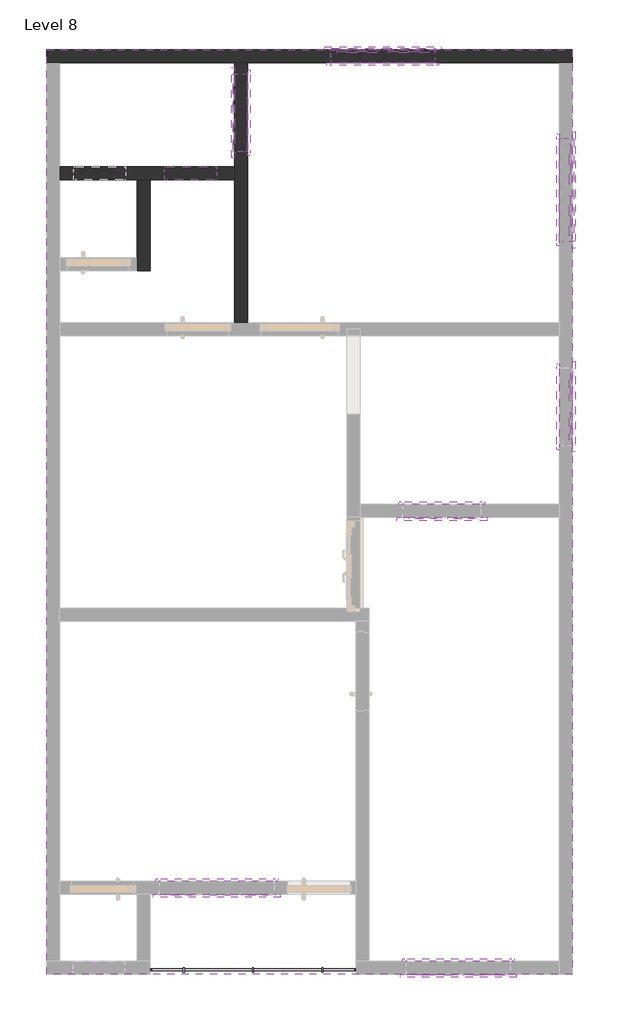
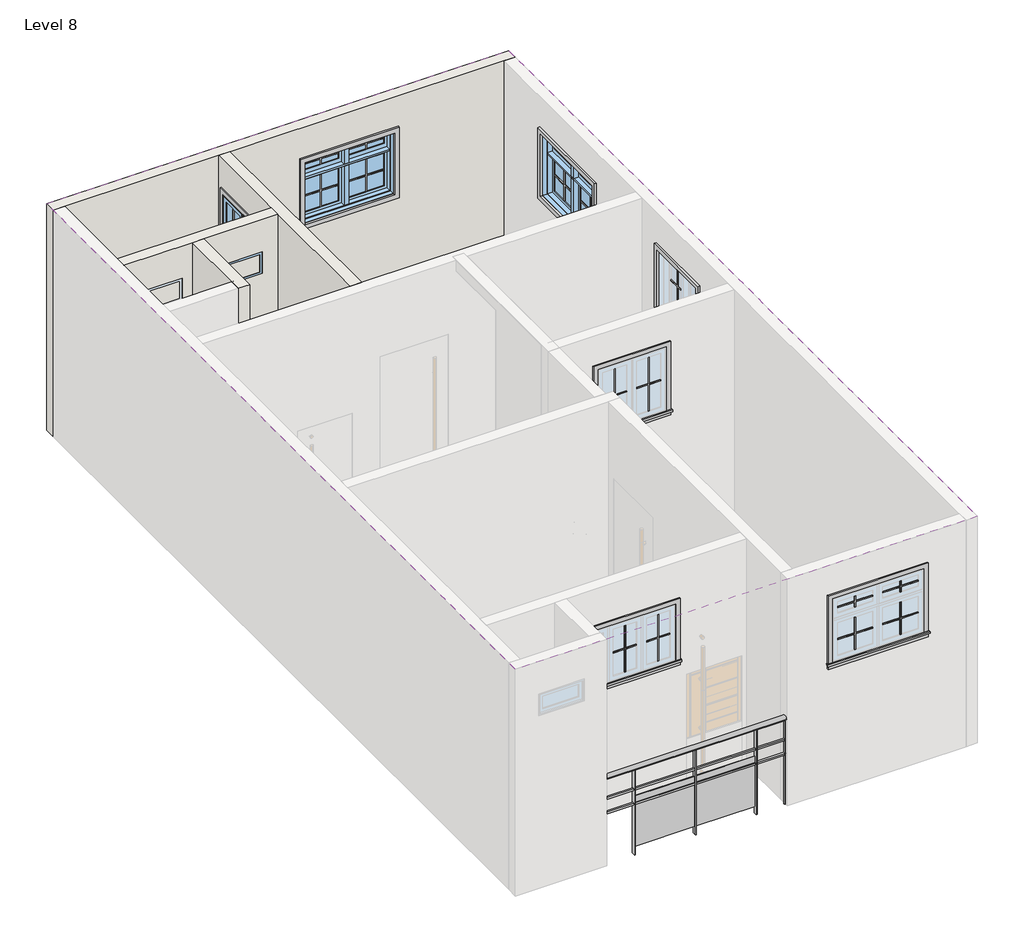
# One storey, part 2 of 2: 48 proxies, 7 walls, 5 windows, 1 covering, 1 railing.
"""IFC4 building model written with IfcOpenShell, lengths in millimetres."""

from ifc_helpers import new_model, si_unit, point, frame, origin, place, context, project, spatial, polyline, ellipse_curve, trimmed, outline, extrude, faceted_brep, transform, mapped, element, save
from ifc_brep_helpers import plane_surface, extruded_surface, advanced_brep
from components import m_muntin_pattern_2x2_m_muntin_pattern_2x2_ec2ff75e, m_muntin_pattern_2x2_m_muntin_pattern_2x2_6a19bea2, m_muntin_pattern_2x2_m_muntin_pattern_2x2_383df7b3, m_muntin_pattern_2x2_m_muntin_pattern_2x2_55460d9e, m_muntin_pattern_2x2_m_muntin_pattern_2x2_a9b7b7a9, m_muntin_pattern_2x2_m_muntin_pattern_2x2_c959817e, m_muntin_pattern_2x2_m_muntin_pattern_2x2_9259c5e2, m_trim_window_exterior_flat_with_sill_b1b88069, m_trim_window_exterior_flat_with_sill_8fa486dc, m_trim_window_exterior_flat_with_sill_2a9c44ae, m_trim_window_interior_flat_picture_frame_7d12f20c, m_trim_window_interior_flat_picture_frame_b6dd03a6, m_trim_window_interior_flat_picture_frame_c139440e, fixed_2_65c13adb, m_window_casement_double_3_e0bd8fa3, m_window_casement_double_awning_double_4_7efa9bbd

model = new_model("IFC4")

# Units and contexts
model_context = context("Model", 3, world=origin())
ifc_project = project(units=[si_unit("LENGTHUNIT", "METRE", prefix="MILLI")], contexts=[model_context])

# Site, building, storey
site = spatial("IfcSite", under=ifc_project)
building = spatial("IfcBuilding", under=site)
storey = spatial("IfcBuildingStorey", under=building, Name="Level 8", Elevation=13411.2)

# Proxies
placement = place(None, origin())
m_muntin_pattern_2x2_m_muntin_pattern_2x2_shape = m_muntin_pattern_2x2_m_muntin_pattern_2x2_ec2ff75e(model_context)
element("IfcBuildingElementProxy", 1, Name="M_Muntin Pattern_2x2 : M_Muntin Pattern_2x2", ObjectType="M_Muntin Pattern_2x2 : M_Muntin Pattern_2x2", at=placement, inside=storey, context=model_context, shape_type="MappedRepresentation", body=[
    mapped(m_muntin_pattern_2x2_m_muntin_pattern_2x2_shape, transform((-20164.8088079, 6316.5492053, 15309.85), x_axis=(1.0, 0.0, 0.0), y_axis=(0.0, 1.0, 0.0), z_axis=(0.0, 0.0, 1.0))),
])
element("IfcBuildingElementProxy", 2, Name="M_Muntin Pattern_2x2 : M_Muntin Pattern_2x2", ObjectType="M_Muntin Pattern_2x2 : M_Muntin Pattern_2x2", at=placement, inside=storey, context=model_context, shape_type="MappedRepresentation", body=[
    mapped(m_muntin_pattern_2x2_m_muntin_pattern_2x2_shape, transform((-17648.6213079, 4984.6367053, 15309.85), x_axis=(0.0, -1.0, 0.0), y_axis=(1.0, 0.0, 0.0), z_axis=(0.0, 0.0, 1.0))),
])
element("IfcBuildingElementProxy", 3, Name="M_Muntin Pattern_2x2 : M_Muntin Pattern_2x2", ObjectType="M_Muntin Pattern_2x2 : M_Muntin Pattern_2x2", at=placement, inside=storey, context=model_context, shape_type="MappedRepresentation", body=[
    mapped(m_muntin_pattern_2x2_m_muntin_pattern_2x2_shape, transform((-18672.7572454, -4510.2007947, 15309.85), x_axis=(-1.0, 0.0, 0.0), y_axis=(0.0, -1.0, 0.0), z_axis=(0.0, 0.0, 1.0))),
])
m_muntin_pattern_2x2_m_muntin_pattern_2x2_2_shape = m_muntin_pattern_2x2_m_muntin_pattern_2x2_6a19bea2(model_context)
element("IfcBuildingElementProxy", 4, Name="M_Muntin Pattern_2x2 : M_Muntin Pattern_2x2", ObjectType="M_Muntin Pattern_2x2 : M_Muntin Pattern_2x2", at=placement, inside=storey, context=model_context, shape_type="MappedRepresentation", body=[
    mapped(m_muntin_pattern_2x2_m_muntin_pattern_2x2_2_shape, transform((-19558.3838079, 6316.5492053, 15309.85), x_axis=(-1.0, 0.0, 0.0), y_axis=(0.0, -1.0, 0.0), z_axis=(0.0, 0.0, 1.0))),
])
element("IfcBuildingElementProxy", 5, Name="M_Muntin Pattern_2x2 : M_Muntin Pattern_2x2", ObjectType="M_Muntin Pattern_2x2 : M_Muntin Pattern_2x2", at=placement, inside=storey, context=model_context, shape_type="MappedRepresentation", body=[
    mapped(m_muntin_pattern_2x2_m_muntin_pattern_2x2_2_shape, transform((-17648.6213079, 4378.2117053, 15309.85), x_axis=(0.0, 1.0, 0.0), y_axis=(-1.0, 0.0, 0.0), z_axis=(0.0, 0.0, 1.0))),
])
element("IfcBuildingElementProxy", 6, Name="M_Muntin Pattern_2x2 : M_Muntin Pattern_2x2", ObjectType="M_Muntin Pattern_2x2 : M_Muntin Pattern_2x2", at=placement, inside=storey, context=model_context, shape_type="MappedRepresentation", body=[
    mapped(m_muntin_pattern_2x2_m_muntin_pattern_2x2_2_shape, transform((-19279.1822454, -4510.2007947, 15309.85), x_axis=(1.0, 0.0, 0.0), y_axis=(0.0, 1.0, 0.0), z_axis=(0.0, 0.0, 1.0))),
])
m_muntin_pattern_2x2_m_muntin_pattern_2x2_3_shape = m_muntin_pattern_2x2_m_muntin_pattern_2x2_383df7b3(model_context)
element("IfcBuildingElementProxy", 7, Name="M_Muntin Pattern_2x2 : M_Muntin Pattern_2x2", ObjectType="M_Muntin Pattern_2x2 : M_Muntin Pattern_2x2", at=placement, inside=storey, context=model_context, shape_type="MappedRepresentation", body=[
    mapped(m_muntin_pattern_2x2_m_muntin_pattern_2x2_3_shape, transform((-19558.3838079, 6316.5492053, 15909.85), x_axis=(-1.0, 0.0, 0.0), y_axis=(0.0, -1.0, 0.0), z_axis=(0.0, 0.0, 1.0))),
])
element("IfcBuildingElementProxy", 8, Name="M_Muntin Pattern_2x2 : M_Muntin Pattern_2x2", ObjectType="M_Muntin Pattern_2x2 : M_Muntin Pattern_2x2", at=placement, inside=storey, context=model_context, shape_type="MappedRepresentation", body=[
    mapped(m_muntin_pattern_2x2_m_muntin_pattern_2x2_3_shape, transform((-20164.8088079, 6316.5492053, 15909.85), x_axis=(-1.0, 0.0, 0.0), y_axis=(0.0, -1.0, 0.0), z_axis=(0.0, 0.0, 1.0))),
])
element("IfcBuildingElementProxy", 9, Name="M_Muntin Pattern_2x2 : M_Muntin Pattern_2x2", ObjectType="M_Muntin Pattern_2x2 : M_Muntin Pattern_2x2", at=placement, inside=storey, context=model_context, shape_type="MappedRepresentation", body=[
    mapped(m_muntin_pattern_2x2_m_muntin_pattern_2x2_3_shape, transform((-17648.6213079, 4378.2117053, 15909.85), x_axis=(0.0, 1.0, 0.0), y_axis=(-1.0, 0.0, 0.0), z_axis=(0.0, 0.0, 1.0))),
])
element("IfcBuildingElementProxy", 10, Name="M_Muntin Pattern_2x2 : M_Muntin Pattern_2x2", ObjectType="M_Muntin Pattern_2x2 : M_Muntin Pattern_2x2", at=placement, inside=storey, context=model_context, shape_type="MappedRepresentation", body=[
    mapped(m_muntin_pattern_2x2_m_muntin_pattern_2x2_3_shape, transform((-17648.6213079, 4984.6367053, 15909.85), x_axis=(0.0, 1.0, 0.0), y_axis=(-1.0, 0.0, 0.0), z_axis=(0.0, 0.0, 1.0))),
])
element("IfcBuildingElementProxy", 11, Name="M_Muntin Pattern_2x2 : M_Muntin Pattern_2x2", ObjectType="M_Muntin Pattern_2x2 : M_Muntin Pattern_2x2", at=placement, inside=storey, context=model_context, shape_type="MappedRepresentation", body=[
    mapped(m_muntin_pattern_2x2_m_muntin_pattern_2x2_3_shape, transform((-19279.1822454, -4510.2007947, 15909.85), x_axis=(1.0, 0.0, 0.0), y_axis=(0.0, 1.0, 0.0), z_axis=(0.0, 0.0, 1.0))),
])
element("IfcBuildingElementProxy", 12, Name="M_Muntin Pattern_2x2 : M_Muntin Pattern_2x2", ObjectType="M_Muntin Pattern_2x2 : M_Muntin Pattern_2x2", at=placement, inside=storey, context=model_context, shape_type="MappedRepresentation", body=[
    mapped(m_muntin_pattern_2x2_m_muntin_pattern_2x2_3_shape, transform((-18672.7572454, -4510.2007947, 15909.85), x_axis=(1.0, 0.0, 0.0), y_axis=(0.0, 1.0, 0.0), z_axis=(0.0, 0.0, 1.0))),
])
m_muntin_pattern_2x2_m_muntin_pattern_2x2_4_shape = m_muntin_pattern_2x2_m_muntin_pattern_2x2_55460d9e(model_context)
element("IfcBuildingElementProxy", 13, Name="M_Muntin Pattern_2x2 : M_Muntin Pattern_2x2", ObjectType="M_Muntin Pattern_2x2 : M_Muntin Pattern_2x2", at=placement, inside=storey, context=model_context, shape_type="MappedRepresentation", body=[
    mapped(m_muntin_pattern_2x2_m_muntin_pattern_2x2_4_shape, transform((-18939.9533391, 849.1992053, 15309.85), x_axis=(-1.0, 0.0, 0.0), y_axis=(0.0, -1.0, 0.0), z_axis=(0.0, 0.0, 1.0))),
])
element("IfcBuildingElementProxy", 14, Name="M_Muntin Pattern_2x2 : M_Muntin Pattern_2x2", ObjectType="M_Muntin Pattern_2x2 : M_Muntin Pattern_2x2", at=placement, inside=storey, context=model_context, shape_type="MappedRepresentation", body=[
    mapped(m_muntin_pattern_2x2_m_muntin_pattern_2x2_4_shape, transform((-17648.6213079, 2366.8492053, 15309.85), x_axis=(0.0, -1.0, 0.0), y_axis=(1.0, 0.0, 0.0), z_axis=(0.0, 0.0, 1.0))),
])
element("IfcBuildingElementProxy", 15, Name="M_Muntin Pattern_2x2 : M_Muntin Pattern_2x2", ObjectType="M_Muntin Pattern_2x2 : M_Muntin Pattern_2x2", at=placement, inside=storey, context=model_context, shape_type="MappedRepresentation", body=[
    mapped(m_muntin_pattern_2x2_m_muntin_pattern_2x2_4_shape, transform((-21591.9713079, 5362.4617053, 15309.85), x_axis=(0.0, 1.0, 0.0), y_axis=(-1.0, 0.0, 0.0), z_axis=(0.0, 0.0, 1.0))),
])
element("IfcBuildingElementProxy", 16, Name="M_Muntin Pattern_2x2 : M_Muntin Pattern_2x2", ObjectType="M_Muntin Pattern_2x2 : M_Muntin Pattern_2x2", at=placement, inside=storey, context=model_context, shape_type="MappedRepresentation", body=[
    mapped(m_muntin_pattern_2x2_m_muntin_pattern_2x2_4_shape, transform((-18939.9533391, 849.1992053, 15309.85), x_axis=(-1.0, 0.0, 0.0), y_axis=(0.0, -1.0, 0.0), z_axis=(0.0, 0.0, 1.0))),
])
element("IfcBuildingElementProxy", 17, Name="M_Muntin Pattern_2x2 : M_Muntin Pattern_2x2", ObjectType="M_Muntin Pattern_2x2 : M_Muntin Pattern_2x2", at=placement, inside=storey, context=model_context, shape_type="MappedRepresentation", body=[
    mapped(m_muntin_pattern_2x2_m_muntin_pattern_2x2_4_shape, transform((-21591.9713079, 5362.4617053, 15309.85), x_axis=(0.0, 1.0, 0.0), y_axis=(-1.0, 0.0, 0.0), z_axis=(0.0, 0.0, 1.0))),
])
m_muntin_pattern_2x2_m_muntin_pattern_2x2_5_shape = m_muntin_pattern_2x2_m_muntin_pattern_2x2_a9b7b7a9(model_context)
element("IfcBuildingElementProxy", 18, Name="M_Muntin Pattern_2x2 : M_Muntin Pattern_2x2", ObjectType="M_Muntin Pattern_2x2 : M_Muntin Pattern_2x2", at=placement, inside=storey, context=model_context, shape_type="MappedRepresentation", body=[
    mapped(m_muntin_pattern_2x2_m_muntin_pattern_2x2_5_shape, transform((-19393.9783391, 849.1992053, 15309.85), x_axis=(1.0, 0.0, 0.0), y_axis=(0.0, 1.0, 0.0), z_axis=(0.0, 0.0, 1.0))),
])
element("IfcBuildingElementProxy", 19, Name="M_Muntin Pattern_2x2 : M_Muntin Pattern_2x2", ObjectType="M_Muntin Pattern_2x2 : M_Muntin Pattern_2x2", at=placement, inside=storey, context=model_context, shape_type="MappedRepresentation", body=[
    mapped(m_muntin_pattern_2x2_m_muntin_pattern_2x2_5_shape, transform((-17648.6213079, 1912.8242053, 15309.85), x_axis=(0.0, 1.0, 0.0), y_axis=(-1.0, 0.0, 0.0), z_axis=(0.0, 0.0, 1.0))),
])
element("IfcBuildingElementProxy", 20, Name="M_Muntin Pattern_2x2 : M_Muntin Pattern_2x2", ObjectType="M_Muntin Pattern_2x2 : M_Muntin Pattern_2x2", at=placement, inside=storey, context=model_context, shape_type="MappedRepresentation", body=[
    mapped(m_muntin_pattern_2x2_m_muntin_pattern_2x2_5_shape, transform((-21591.9713079, 5816.4867053, 15309.85), x_axis=(0.0, -1.0, 0.0), y_axis=(1.0, 0.0, 0.0), z_axis=(0.0, 0.0, 1.0))),
])
element("IfcBuildingElementProxy", 21, Name="M_Muntin Pattern_2x2 : M_Muntin Pattern_2x2", ObjectType="M_Muntin Pattern_2x2 : M_Muntin Pattern_2x2", at=placement, inside=storey, context=model_context, shape_type="MappedRepresentation", body=[
    mapped(m_muntin_pattern_2x2_m_muntin_pattern_2x2_5_shape, transform((-19393.9783391, 849.1992053, 15309.85), x_axis=(1.0, 0.0, 0.0), y_axis=(0.0, 1.0, 0.0), z_axis=(0.0, 0.0, 1.0))),
])
element("IfcBuildingElementProxy", 22, Name="M_Muntin Pattern_2x2 : M_Muntin Pattern_2x2", ObjectType="M_Muntin Pattern_2x2 : M_Muntin Pattern_2x2", at=placement, inside=storey, context=model_context, shape_type="MappedRepresentation", body=[
    mapped(m_muntin_pattern_2x2_m_muntin_pattern_2x2_5_shape, transform((-21591.9713079, 5816.4867053, 15309.85), x_axis=(0.0, -1.0, 0.0), y_axis=(1.0, 0.0, 0.0), z_axis=(0.0, 0.0, 1.0))),
])
m_muntin_pattern_2x2_m_muntin_pattern_2x2_6_shape = m_muntin_pattern_2x2_m_muntin_pattern_2x2_c959817e(model_context)
element("IfcBuildingElementProxy", 23, Name="M_Muntin Pattern_2x2 : M_Muntin Pattern_2x2", ObjectType="M_Muntin Pattern_2x2 : M_Muntin Pattern_2x2", at=placement, inside=storey, context=model_context, shape_type="MappedRepresentation", body=[
    mapped(m_muntin_pattern_2x2_m_muntin_pattern_2x2_6_shape, transform((-21364.4296412, -3570.4007947, 15309.85), x_axis=(-1.0, 0.0, 0.0), y_axis=(0.0, -1.0, 0.0), z_axis=(0.0, 0.0, 1.0))),
])
element("IfcBuildingElementProxy", 24, Name="M_Muntin Pattern_2x2 : M_Muntin Pattern_2x2", ObjectType="M_Muntin Pattern_2x2 : M_Muntin Pattern_2x2", at=placement, inside=storey, context=model_context, shape_type="MappedRepresentation", body=[
    mapped(m_muntin_pattern_2x2_m_muntin_pattern_2x2_6_shape, transform((-21364.4296412, -3570.4007947, 15309.85), x_axis=(-1.0, 0.0, 0.0), y_axis=(0.0, -1.0, 0.0), z_axis=(0.0, 0.0, 1.0))),
])
m_muntin_pattern_2x2_m_muntin_pattern_2x2_7_shape = m_muntin_pattern_2x2_m_muntin_pattern_2x2_9259c5e2(model_context)
element("IfcBuildingElementProxy", 25, Name="M_Muntin Pattern_2x2 : M_Muntin Pattern_2x2", ObjectType="M_Muntin Pattern_2x2 : M_Muntin Pattern_2x2", at=placement, inside=storey, context=model_context, shape_type="MappedRepresentation", body=[
    mapped(m_muntin_pattern_2x2_m_muntin_pattern_2x2_7_shape, transform((-22257.6629746, -3570.4007947, 15309.85), x_axis=(1.0, 0.0, 0.0), y_axis=(0.0, 1.0, 0.0), z_axis=(0.0, 0.0, 1.0))),
])
element("IfcBuildingElementProxy", 26, Name="M_Muntin Pattern_2x2 : M_Muntin Pattern_2x2", ObjectType="M_Muntin Pattern_2x2 : M_Muntin Pattern_2x2", at=placement, inside=storey, context=model_context, shape_type="MappedRepresentation", body=[
    mapped(m_muntin_pattern_2x2_m_muntin_pattern_2x2_7_shape, transform((-21811.0463079, -3570.4007947, 15309.85), x_axis=(1.0, 0.0, 0.0), y_axis=(0.0, 1.0, 0.0), z_axis=(0.0, 0.0, 1.0))),
])
element("IfcBuildingElementProxy", 27, Name="M_Muntin Pattern_2x2 : M_Muntin Pattern_2x2", ObjectType="M_Muntin Pattern_2x2 : M_Muntin Pattern_2x2", at=placement, inside=storey, context=model_context, shape_type="MappedRepresentation", body=[
    mapped(m_muntin_pattern_2x2_m_muntin_pattern_2x2_7_shape, transform((-22257.6629746, -3570.4007947, 15309.85), x_axis=(1.0, 0.0, 0.0), y_axis=(0.0, 1.0, 0.0), z_axis=(0.0, 0.0, 1.0))),
])
element("IfcBuildingElementProxy", 28, Name="M_Muntin Pattern_2x2 : M_Muntin Pattern_2x2", ObjectType="M_Muntin Pattern_2x2 : M_Muntin Pattern_2x2", at=placement, inside=storey, context=model_context, shape_type="MappedRepresentation", body=[
    mapped(m_muntin_pattern_2x2_m_muntin_pattern_2x2_7_shape, transform((-21811.0463079, -3570.4007947, 15309.85), x_axis=(1.0, 0.0, 0.0), y_axis=(0.0, 1.0, 0.0), z_axis=(0.0, 0.0, 1.0))),
])
m_trim_window_exterior_flat_with_sill_shape = m_trim_window_exterior_flat_with_sill_b1b88069(model_context)
element("IfcBuildingElementProxy", 29, Name="M_Trim-Window-Exterior-Flat : with Sill", ObjectType="M_Trim-Window-Exterior-Flat : with Sill", at=placement, inside=storey, context=model_context, shape_type="MappedRepresentation", body=[
    mapped(m_trim_window_exterior_flat_with_sill_shape, transform((-19861.5963079, 6326.0742053, 16140.0), x_axis=(-1.0, 0.0, 0.0), y_axis=(0.0, 0.0, 1.0), z_axis=(0.0, 1.0, 0.0))),
])
element("IfcBuildingElementProxy", 30, Name="M_Trim-Window-Exterior-Flat : with Sill", ObjectType="M_Trim-Window-Exterior-Flat : with Sill", at=placement, inside=storey, context=model_context, shape_type="MappedRepresentation", body=[
    mapped(m_trim_window_exterior_flat_with_sill_shape, transform((-17639.0963079, 4681.4242053, 16140.0), x_axis=(0.0, 1.0, 0.0), y_axis=(0.0, 0.0, 1.0), z_axis=(1.0, 0.0, 0.0))),
])
element("IfcBuildingElementProxy", 31, Name="M_Trim-Window-Exterior-Flat : with Sill", ObjectType="M_Trim-Window-Exterior-Flat : with Sill", at=placement, inside=storey, context=model_context, shape_type="MappedRepresentation", body=[
    mapped(m_trim_window_exterior_flat_with_sill_shape, transform((-18975.9697454, -4519.7257947, 16140.0), x_axis=(1.0, 0.0, 0.0), y_axis=(0.0, 0.0, 1.0), z_axis=(0.0, -1.0, 0.0))),
])
m_trim_window_exterior_flat_with_sill_2_shape = m_trim_window_exterior_flat_with_sill_8fa486dc(model_context)
element("IfcBuildingElementProxy", 32, Name="M_Trim-Window-Exterior-Flat : with Sill", ObjectType="M_Trim-Window-Exterior-Flat : with Sill", at=placement, inside=storey, context=model_context, shape_type="MappedRepresentation", body=[
    mapped(m_trim_window_exterior_flat_with_sill_2_shape, transform((-19166.9658391, 839.6742053, 16140.0), x_axis=(1.0, 0.0, 0.0), y_axis=(0.0, 0.0, 1.0), z_axis=(0.0, -1.0, 0.0))),
])
element("IfcBuildingElementProxy", 33, Name="M_Trim-Window-Exterior-Flat : with Sill", ObjectType="M_Trim-Window-Exterior-Flat : with Sill", at=placement, inside=storey, context=model_context, shape_type="MappedRepresentation", body=[
    mapped(m_trim_window_exterior_flat_with_sill_2_shape, transform((-17639.0963079, 2139.8367053, 16140.0), x_axis=(0.0, 1.0, 0.0), y_axis=(0.0, 0.0, 1.0), z_axis=(1.0, 0.0, 0.0))),
])
element("IfcBuildingElementProxy", 34, Name="M_Trim-Window-Exterior-Flat : with Sill", ObjectType="M_Trim-Window-Exterior-Flat : with Sill", at=placement, inside=storey, context=model_context, shape_type="MappedRepresentation", body=[
    mapped(m_trim_window_exterior_flat_with_sill_2_shape, transform((-21601.4963079, 5589.4742053, 16140.0), x_axis=(0.0, -1.0, 0.0), y_axis=(0.0, 0.0, 1.0), z_axis=(-1.0, 0.0, 0.0))),
])
element("IfcBuildingElementProxy", 35, Name="M_Trim-Window-Exterior-Flat : with Sill", ObjectType="M_Trim-Window-Exterior-Flat : with Sill", at=placement, inside=storey, context=model_context, shape_type="MappedRepresentation", body=[
    mapped(m_trim_window_exterior_flat_with_sill_2_shape, transform((-19166.9658391, 839.6742053, 16140.0), x_axis=(1.0, 0.0, 0.0), y_axis=(0.0, 0.0, 1.0), z_axis=(0.0, -1.0, 0.0))),
])
element("IfcBuildingElementProxy", 36, Name="M_Trim-Window-Exterior-Flat : with Sill", ObjectType="M_Trim-Window-Exterior-Flat : with Sill", at=placement, inside=storey, context=model_context, shape_type="MappedRepresentation", body=[
    mapped(m_trim_window_exterior_flat_with_sill_2_shape, transform((-21601.4963079, 5589.4742053, 16140.0), x_axis=(0.0, -1.0, 0.0), y_axis=(0.0, 0.0, 1.0), z_axis=(-1.0, 0.0, 0.0))),
])
m_trim_window_exterior_flat_with_sill_3_shape = m_trim_window_exterior_flat_with_sill_2a9c44ae(model_context)
element("IfcBuildingElementProxy", 37, Name="M_Trim-Window-Exterior-Flat : with Sill", ObjectType="M_Trim-Window-Exterior-Flat : with Sill", at=placement, inside=storey, context=model_context, shape_type="MappedRepresentation", body=[
    mapped(m_trim_window_exterior_flat_with_sill_3_shape, transform((-21811.0463079, -3579.9257947, 16040.0), x_axis=(1.0, 0.0, 0.0), y_axis=(0.0, 0.0, 1.0), z_axis=(0.0, -1.0, 0.0))),
])
element("IfcBuildingElementProxy", 38, Name="M_Trim-Window-Exterior-Flat : with Sill", ObjectType="M_Trim-Window-Exterior-Flat : with Sill", at=placement, inside=storey, context=model_context, shape_type="MappedRepresentation", body=[
    mapped(m_trim_window_exterior_flat_with_sill_3_shape, transform((-21811.0463079, -3579.9257947, 16040.0), x_axis=(1.0, 0.0, 0.0), y_axis=(0.0, 0.0, 1.0), z_axis=(0.0, -1.0, 0.0))),
])
m_trim_window_interior_flat_picture_frame_shape = m_trim_window_interior_flat_picture_frame_7d12f20c(model_context)
element("IfcBuildingElementProxy", 39, Name="M_Trim-Window-Interior-Flat : Picture Frame", ObjectType="M_Trim-Window-Interior-Flat : Picture Frame", at=placement, inside=storey, context=model_context, shape_type="MappedRepresentation", body=[
    mapped(m_trim_window_interior_flat_picture_frame_shape, transform((-19861.5963079, 6173.6742053, 16140.0), x_axis=(1.0, 0.0, 0.0), y_axis=(0.0, 0.0, 1.0), z_axis=(0.0, -1.0, 0.0))),
])
element("IfcBuildingElementProxy", 40, Name="M_Trim-Window-Interior-Flat : Picture Frame", ObjectType="M_Trim-Window-Interior-Flat : Picture Frame", at=placement, inside=storey, context=model_context, shape_type="MappedRepresentation", body=[
    mapped(m_trim_window_interior_flat_picture_frame_shape, transform((-17791.4963079, 4681.4242053, 16140.0), x_axis=(0.0, -1.0, 0.0), y_axis=(0.0, 0.0, 1.0), z_axis=(-1.0, 0.0, 0.0))),
])
element("IfcBuildingElementProxy", 41, Name="M_Trim-Window-Interior-Flat : Picture Frame", ObjectType="M_Trim-Window-Interior-Flat : Picture Frame", at=placement, inside=storey, context=model_context, shape_type="MappedRepresentation", body=[
    mapped(m_trim_window_interior_flat_picture_frame_shape, transform((-18975.9697454, -4367.3257947, 16140.0), x_axis=(-1.0, 0.0, 0.0), y_axis=(0.0, 0.0, 1.0), z_axis=(0.0, 1.0, 0.0))),
])
m_trim_window_interior_flat_picture_frame_2_shape = m_trim_window_interior_flat_picture_frame_b6dd03a6(model_context)
element("IfcBuildingElementProxy", 42, Name="M_Trim-Window-Interior-Flat : Picture Frame", ObjectType="M_Trim-Window-Interior-Flat : Picture Frame", at=placement, inside=storey, context=model_context, shape_type="MappedRepresentation", body=[
    mapped(m_trim_window_interior_flat_picture_frame_2_shape, transform((-19166.9658391, 992.0742053, 16140.0), x_axis=(-1.0, 0.0, 0.0), y_axis=(0.0, 0.0, 1.0), z_axis=(0.0, 1.0, 0.0))),
])
element("IfcBuildingElementProxy", 43, Name="M_Trim-Window-Interior-Flat : Picture Frame", ObjectType="M_Trim-Window-Interior-Flat : Picture Frame", at=placement, inside=storey, context=model_context, shape_type="MappedRepresentation", body=[
    mapped(m_trim_window_interior_flat_picture_frame_2_shape, transform((-17791.4963079, 2139.8367053, 16140.0), x_axis=(0.0, -1.0, 0.0), y_axis=(0.0, 0.0, 1.0), z_axis=(-1.0, 0.0, 0.0))),
])
element("IfcBuildingElementProxy", 44, Name="M_Trim-Window-Interior-Flat : Picture Frame", ObjectType="M_Trim-Window-Interior-Flat : Picture Frame", at=placement, inside=storey, context=model_context, shape_type="MappedRepresentation", body=[
    mapped(m_trim_window_interior_flat_picture_frame_2_shape, transform((-21449.0963079, 5589.4742053, 16140.0), x_axis=(0.0, 1.0, 0.0), y_axis=(0.0, 0.0, 1.0), z_axis=(1.0, 0.0, 0.0))),
])
element("IfcBuildingElementProxy", 45, Name="M_Trim-Window-Interior-Flat : Picture Frame", ObjectType="M_Trim-Window-Interior-Flat : Picture Frame", at=placement, inside=storey, context=model_context, shape_type="MappedRepresentation", body=[
    mapped(m_trim_window_interior_flat_picture_frame_2_shape, transform((-19166.9658391, 992.0742053, 16140.0), x_axis=(-1.0, 0.0, 0.0), y_axis=(0.0, 0.0, 1.0), z_axis=(0.0, 1.0, 0.0))),
])
element("IfcBuildingElementProxy", 46, Name="M_Trim-Window-Interior-Flat : Picture Frame", ObjectType="M_Trim-Window-Interior-Flat : Picture Frame", at=placement, inside=storey, context=model_context, shape_type="MappedRepresentation", body=[
    mapped(m_trim_window_interior_flat_picture_frame_2_shape, transform((-21449.0963079, 5589.4742053, 16140.0), x_axis=(0.0, 1.0, 0.0), y_axis=(0.0, 0.0, 1.0), z_axis=(1.0, 0.0, 0.0))),
])
m_trim_window_interior_flat_picture_frame_3_shape = m_trim_window_interior_flat_picture_frame_c139440e(model_context)
element("IfcBuildingElementProxy", 47, Name="M_Trim-Window-Interior-Flat : Picture Frame", ObjectType="M_Trim-Window-Interior-Flat : Picture Frame", at=placement, inside=storey, context=model_context, shape_type="MappedRepresentation", body=[
    mapped(m_trim_window_interior_flat_picture_frame_3_shape, transform((-21811.0463079, -3427.5257947, 16040.0), x_axis=(-1.0, 0.0, 0.0), y_axis=(0.0, 0.0, 1.0), z_axis=(0.0, 1.0, 0.0))),
])
element("IfcBuildingElementProxy", 48, Name="M_Trim-Window-Interior-Flat : Picture Frame", ObjectType="M_Trim-Window-Interior-Flat : Picture Frame", at=placement, inside=storey, context=model_context, shape_type="MappedRepresentation", body=[
    mapped(m_trim_window_interior_flat_picture_frame_3_shape, transform((-21811.0463079, -3427.5257947, 16040.0), x_axis=(-1.0, 0.0, 0.0), y_axis=(0.0, 0.0, 1.0), z_axis=(0.0, 1.0, 0.0))),
])

# Covering
element("IfcCovering", 49, ObjectType="2' x 4' ACT System", at=placement, inside=storey, context=model_context, shape_type="SweptSolid", body=[
    extrude(outline(polyline([(-23811.2963079, -4519.7257947), (-23811.2963079, 6326.0742053), (-17639.0963079, 6326.0742053), (-17639.0963079, -4519.7257947), (-22309.2664727, -4519.7257947), (-23811.2963079, -4519.7257947)])), frame((0.0, 0.0, 16611.6), z_axis=(0.0, 0.0, 1.0), x_axis=(1.0, 0.0, 0.0)), (0.0, 0.0, 1.0), 57.15),
])

# Railing
element("IfcRailing", 50, ObjectType="Glass Panel - Bottom Fill", at=placement, inside=storey, context=model_context, shape_type="SolidModel", body=[
    advanced_brep(
    [(-22592.0963079, -4430.8257947, 14630.4), (-22592.0963079, -4507.0257947, 14630.4), (-20179.0963079, -4430.8257947, 14630.4), (-20179.0963079, -4507.0257947, 14630.4)],
    [
        (0, 1, ellipse_curve(frame((-22592.0963079, -4468.9257947, 14630.4), z_axis=(-1.0, 0.0, 0.0), x_axis=(0.0, -1.0, 0.0)), 38.1, 28.575)),
        (1, 0, ellipse_curve(frame((-22592.0963079, -4468.9257947, 14630.4), z_axis=(-1.0, 0.0, 0.0), x_axis=(0.0, -1.0, 0.0)), 38.1, 28.575)),
        (2, 3, ellipse_curve(frame((-20179.0963079, -4468.9257947, 14630.4), z_axis=(1.0, 0.0, 0.0), x_axis=(0.0, -1.0, 0.0)), 38.1, 28.575)),
        (3, 2, ellipse_curve(frame((-20179.0963079, -4468.9257947, 14630.4), z_axis=(1.0, 0.0, 0.0), x_axis=(0.0, -1.0, 0.0)), 38.1, 28.575)),
        (0, 2),
        (3, 1),
    ],
    [
        plane_surface(frame((-22592.0963079, -4468.9257947, 14630.4), z_axis=(-1.0, 0.0, 0.0), x_axis=(0.0, 1.0, 0.0))),
        plane_surface(frame((-20179.0963079, -4468.9257947, 14630.4), z_axis=(1.0, 0.0, 0.0), x_axis=(0.0, 1.0, 0.0))),
        extruded_surface(trimmed(ellipse_curve(frame((-20179.0963079, -4468.9257947, 14630.4), z_axis=(-1.0, 0.0, 0.0), x_axis=(0.0, -1.0, 0.0)), 38.1, 28.575), [point((-20179.0963079, -4430.8257947, 14630.4))], [point((-20179.0963079, -4507.0257947, 14630.4))], True, "CARTESIAN"), (-2413.0, 0.0, 0.0), 2413.0),
        extruded_surface(trimmed(ellipse_curve(frame((-20179.0963079, -4468.9257947, 14630.4), z_axis=(-1.0, 0.0, 0.0), x_axis=(0.0, -1.0, 0.0)), 38.1, 28.575), [point((-20179.0963079, -4507.0257947, 14630.4))], [point((-20179.0963079, -4430.8257947, 14630.4))], True, "CARTESIAN"), (-2413.0, 0.0, 0.0), 2413.0),
    ],
    [
        (0, [[1, 2]]),
        (1, [[3, 4]]),
        (2, [[-1, 5, -4, 6]]),
        (3, [[-2, -6, -3, -5]]),
    ],
),
    extrude(outline(polyline([(-22592.0963079, -4481.6257947), (-22592.0963079, -4456.2257947), (-20179.0963079, -4456.2257947), (-20179.0963079, -4481.6257947), (-22592.0963079, -4481.6257947)])), frame((0.0, 0.0, 14312.9), z_axis=(0.0, 0.0, 1.0), x_axis=(1.0, 0.0, 0.0)), (0.0, 0.0, 1.0), 25.4),
    extrude(outline(polyline([(-22592.0963079, -4481.6257947), (-22592.0963079, -4456.2257947), (-20179.0963079, -4456.2257947), (-20179.0963079, -4481.6257947), (-22592.0963079, -4481.6257947)])), frame((0.0, 0.0, 14109.7), z_axis=(0.0, 0.0, 1.0), x_axis=(1.0, 0.0, 0.0)), (0.0, 0.0, 1.0), 25.4),
    extrude(outline(polyline([(-20579.1463079, -4494.3257947), (-20579.1463079, -4443.5257947), (-20566.4463079, -4443.5257947), (-20566.4463079, -4494.3257947), (-20579.1463079, -4494.3257947)])), frame((0.0, 0.0, 13411.2), z_axis=(0.0, 0.0, 1.0), x_axis=(1.0, 0.0, 0.0)), (0.0, 0.0, 1.0), 1190.625),
    extrude(outline(polyline([(-21385.5963079, -4462.3906377), (-20572.7963079, -4462.3906377), (-20572.7963079, -4468.7406377), (-21385.5963079, -4468.7406377), (-21385.5963079, -4462.3906377)])), frame((0.0, 0.0, 13512.8), z_axis=(0.0, 0.0, 1.0), x_axis=(1.0, 0.0, 0.0)), (0.0, 0.0, 1.0), 711.2),
    extrude(outline(polyline([(-21391.9463079, -4494.3257947), (-21391.9463079, -4443.5257947), (-21379.2463079, -4443.5257947), (-21379.2463079, -4494.3257947), (-21391.9463079, -4494.3257947)])), frame((0.0, 0.0, 13411.2), z_axis=(0.0, 0.0, 1.0), x_axis=(1.0, 0.0, 0.0)), (0.0, 0.0, 1.0), 1190.625),
    extrude(outline(polyline([(-22198.3963079, -4462.3906377), (-21385.5963079, -4462.3906377), (-21385.5963079, -4468.7406377), (-22198.3963079, -4468.7406377), (-22198.3963079, -4462.3906377)])), frame((0.0, 0.0, 13512.8), z_axis=(0.0, 0.0, 1.0), x_axis=(1.0, 0.0, 0.0)), (0.0, 0.0, 1.0), 711.2),
    extrude(outline(polyline([(-22204.7463079, -4494.3257947), (-22204.7463079, -4443.5257947), (-22192.0463079, -4443.5257947), (-22192.0463079, -4494.3257947), (-22204.7463079, -4494.3257947)])), frame((0.0, 0.0, 13411.2), z_axis=(0.0, 0.0, 1.0), x_axis=(1.0, 0.0, 0.0)), (0.0, 0.0, 1.0), 1190.625),
    extrude(outline(polyline([(-20191.7963079, -4478.4507947), (-20191.7963079, -4459.4007947), (-20172.7463079, -4459.4007947), (-20172.7463079, -4478.4507947), (-20191.7963079, -4478.4507947)])), frame((0.0, 0.0, 13411.2), z_axis=(0.0, 0.0, 1.0), x_axis=(1.0, 0.0, 0.0)), (0.0, 0.0, 1.0), 1190.625),
    extrude(outline(polyline([(-22598.4463079, -4478.4507947), (-22598.4463079, -4459.4007947), (-22579.3963079, -4459.4007947), (-22579.3963079, -4478.4507947), (-22598.4463079, -4478.4507947)])), frame((0.0, 0.0, 13411.2), z_axis=(0.0, 0.0, 1.0), x_axis=(1.0, 0.0, 0.0)), (0.0, 0.0, 1.0), 1190.625),
])

# Walls
element("IfcWall", 51, ObjectType="Generic - 6\"", at=placement, inside=storey, context=model_context, shape_type="Brep", body=[
    faceted_brep([(-23811.2963079, 6173.6742053, 13411.2), (-23658.8963079, 6173.6742053, 13411.2), (-21601.4963079, 6173.6742053, 13411.2), (-21449.0963079, 6173.6742053, 13411.2), (-17791.4963079, 6173.6742053, 13411.2), (-17639.0963079, 6173.6742053, 13411.2), (-17639.0963079, 6173.6742053, 16611.6), (-17791.4963079, 6173.6742053, 16611.6), (-21449.0963079, 6173.6742053, 16611.6), (-21601.4963079, 6173.6742053, 16611.6), (-23658.8963079, 6173.6742053, 16611.6), (-23811.2963079, 6173.6742053, 16611.6), (-19251.9963079, 6173.6742053, 16140.0), (-19251.9963079, 6173.6742053, 15240.0), (-20471.1963079, 6173.6742053, 15240.0), (-20471.1963079, 6173.6742053, 16140.0), (-23811.2963079, 6326.0742053, 13411.2), (-23811.2963079, 6326.0742053, 16611.6), (-17639.0963079, 6326.0742053, 16611.6), (-17639.0963079, 6326.0742053, 13411.2), (-19251.9963079, 6326.0742053, 16140.0), (-20471.1963079, 6326.0742053, 16140.0), (-20471.1963079, 6326.0742053, 15240.0), (-19251.9963079, 6326.0742053, 15240.0)], [[[0, 1, 2, 3, 4, 5, 6, 7, 8, 9, 10, 11], [12, 13, 14, 15]], [[16, 17, 18, 19], [20, 21, 22, 23]], [[5, 4, 3, 2, 1, 0, 16, 19]], [[11, 10, 9, 8, 7, 6, 18, 17]], [[6, 5, 19, 18]], [[0, 11, 17, 16]], [[13, 12, 20, 23]], [[14, 13, 23, 22]], [[15, 14, 22, 21]], [[12, 15, 21, 20]]]),
])
element("IfcWall", 52, ObjectType="Generic - 6\"", at=placement, inside=storey, context=model_context, shape_type="Brep", body=[
    faceted_brep([(-21601.4963079, 6173.6742053, 13411.2), (-21601.4963079, 4954.4742053, 13411.2), (-21601.4963079, 4802.0742053, 13411.2), (-21601.4963079, 3125.6742053, 13411.2), (-21601.4963079, 3125.6742053, 16611.6), (-21601.4963079, 4802.0742053, 16611.6), (-21601.4963079, 4954.4742053, 16611.6), (-21601.4963079, 6173.6742053, 16611.6), (-21601.4963079, 6046.6742053, 16140.0), (-21601.4963079, 5132.2742053, 16140.0), (-21601.4963079, 5132.2742053, 15240.0), (-21601.4963079, 6046.6742053, 15240.0), (-21449.0963079, 6173.6742053, 13411.2), (-21449.0963079, 6173.6742053, 16611.6), (-21449.0963079, 3125.6742053, 16611.6), (-21449.0963079, 3125.6742053, 13411.2), (-21449.0963079, 6046.6742053, 16140.0), (-21449.0963079, 6046.6742053, 15240.0), (-21449.0963079, 5132.2742053, 15240.0), (-21449.0963079, 5132.2742053, 16140.0)], [[[0, 1, 2, 3, 4, 5, 6, 7], [8, 9, 10, 11]], [[12, 13, 14, 15], [16, 17, 18, 19]], [[3, 2, 1, 0, 12, 15]], [[7, 6, 5, 4, 14, 13]], [[0, 7, 13, 12]], [[4, 3, 15, 14]], [[17, 16, 8, 11]], [[18, 17, 11, 10]], [[19, 18, 10, 9]], [[16, 19, 9, 8]]]),
])
element("IfcWall", 53, ObjectType="Generic - 6\"", at=placement, inside=storey, context=model_context, shape_type="Brep", body=[
    faceted_brep([(-23658.8963079, 4802.0742053, 13411.2), (-22744.4963079, 4802.0742053, 13411.2), (-22592.0963079, 4802.0742053, 13411.2), (-21601.4963079, 4802.0742053, 13411.2), (-21601.4963079, 4802.0742053, 16611.6), (-22592.0963079, 4802.0742053, 16611.6), (-22744.4963079, 4802.0742053, 16611.6), (-23658.8963079, 4802.0742053, 16611.6), (-22880.5252141, 4802.0742053, 16154.4), (-22880.5252141, 4802.0742053, 15849.6), (-23490.1252141, 4802.0742053, 15849.6), (-23490.1252141, 4802.0742053, 16154.4), (-21812.6338079, 4802.0742053, 16154.4), (-21812.6338079, 4802.0742053, 15849.6), (-22422.2338079, 4802.0742053, 15849.6), (-22422.2338079, 4802.0742053, 16154.4), (-23658.8963079, 4954.4742053, 13411.2), (-23658.8963079, 4954.4742053, 16611.6), (-21601.4963079, 4954.4742053, 16611.6), (-21601.4963079, 4954.4742053, 13411.2), (-22880.5252141, 4954.4742053, 16154.4), (-23490.1252141, 4954.4742053, 16154.4), (-23490.1252141, 4954.4742053, 15849.6), (-22880.5252141, 4954.4742053, 15849.6), (-21812.6338079, 4954.4742053, 16154.4), (-22422.2338079, 4954.4742053, 16154.4), (-22422.2338079, 4954.4742053, 15849.6), (-21812.6338079, 4954.4742053, 15849.6)], [[[0, 1, 2, 3, 4, 5, 6, 7], [8, 9, 10, 11], [12, 13, 14, 15]], [[16, 17, 18, 19], [20, 21, 22, 23], [24, 25, 26, 27]], [[3, 2, 1, 0, 16, 19]], [[7, 6, 5, 4, 18, 17]], [[0, 7, 17, 16]], [[4, 3, 19, 18]], [[9, 8, 20, 23]], [[10, 9, 23, 22]], [[11, 10, 22, 21]], [[8, 11, 21, 20]], [[13, 12, 24, 27]], [[14, 13, 27, 26]], [[15, 14, 26, 25]], [[12, 15, 25, 24]]]),
])
element("IfcWall", 54, ObjectType="Generic - 6\"", at=placement, inside=storey, context=model_context, shape_type="Brep", body=[
    faceted_brep([(-22744.4963079, 4802.0742053, 13411.2), (-22744.4963079, 3887.6742053, 13411.2), (-22744.4963079, 3735.2742053, 13411.2), (-22744.4963079, 3735.2742053, 16611.6), (-22744.4963079, 3887.6742053, 16611.6), (-22744.4963079, 4802.0742053, 16611.6), (-22592.0963079, 4802.0742053, 13411.2), (-22592.0963079, 4802.0742053, 16611.6), (-22592.0963079, 3735.2742053, 16611.6), (-22592.0963079, 3735.2742053, 13411.2)], [[[0, 1, 2, 3, 4, 5]], [[6, 7, 8, 9]], [[2, 1, 0, 6, 9]], [[5, 4, 3, 8, 7]], [[0, 5, 7, 6]], [[3, 2, 9, 8]]]),
])
element("IfcWall", 55, ObjectType="Generic - 6\"", at=placement, inside=storey, context=model_context, shape_type="Brep", body=[
    faceted_brep([(-21601.4963079, 6173.6742053, 13411.2), (-21601.4963079, 4954.4742053, 13411.2), (-21601.4963079, 4802.0742053, 13411.2), (-21601.4963079, 3125.6742053, 13411.2), (-21601.4963079, 3125.6742053, 16611.6), (-21601.4963079, 4802.0742053, 16611.6), (-21601.4963079, 4954.4742053, 16611.6), (-21601.4963079, 6173.6742053, 16611.6), (-21601.4963079, 6046.6742053, 16140.0), (-21601.4963079, 5132.2742053, 16140.0), (-21601.4963079, 5132.2742053, 15240.0), (-21601.4963079, 6046.6742053, 15240.0), (-21449.0963079, 6173.6742053, 13411.2), (-21449.0963079, 6173.6742053, 16611.6), (-21449.0963079, 3125.6742053, 16611.6), (-21449.0963079, 3125.6742053, 13411.2), (-21449.0963079, 6046.6742053, 16140.0), (-21449.0963079, 6046.6742053, 15240.0), (-21449.0963079, 5132.2742053, 15240.0), (-21449.0963079, 5132.2742053, 16140.0)], [[[0, 1, 2, 3, 4, 5, 6, 7], [8, 9, 10, 11]], [[12, 13, 14, 15], [16, 17, 18, 19]], [[3, 2, 1, 0, 12, 15]], [[7, 6, 5, 4, 14, 13]], [[4, 3, 15, 14]], [[17, 16, 8, 11]], [[18, 17, 11, 10]], [[19, 18, 10, 9]], [[16, 19, 9, 8]], [[0, 7, 13, 12]]]),
])
element("IfcWall", 56, ObjectType="Generic - 6\"", at=placement, inside=storey, context=model_context, shape_type="Brep", body=[
    faceted_brep([(-23658.8963079, 4802.0742053, 13411.2), (-22744.4963079, 4802.0742053, 13411.2), (-22592.0963079, 4802.0742053, 13411.2), (-21601.4963079, 4802.0742053, 13411.2), (-21601.4963079, 4802.0742053, 16611.6), (-22592.0963079, 4802.0742053, 16611.6), (-22744.4963079, 4802.0742053, 16611.6), (-23658.8963079, 4802.0742053, 16611.6), (-23658.8963079, 4954.4742053, 13411.2), (-23658.8963079, 4954.4742053, 16611.6), (-21601.4963079, 4954.4742053, 16611.6), (-21601.4963079, 4954.4742053, 13411.2)], [[[0, 1, 2, 3, 4, 5, 6, 7]], [[8, 9, 10, 11]], [[3, 2, 1, 0, 8, 11]], [[7, 6, 5, 4, 10, 9]], [[4, 3, 11, 10]], [[0, 7, 9, 8]]]),
])
element("IfcWall", 57, ObjectType="Generic - 6\"", at=placement, inside=storey, context=model_context, shape_type="SweptSolid", body=[
    extrude(outline(polyline([(-22744.4963079, 3887.6742053), (-22744.4963079, 4802.0742053), (-22592.0963079, 4802.0742053), (-22592.0963079, 3887.6742053), (-22744.4963079, 3887.6742053)])), frame((0.0, 0.0, 13411.2), z_axis=(0.0, 0.0, 1.0), x_axis=(1.0, 0.0, 0.0)), (0.0, 0.0, 1.0), 3200.4),
])

# Windows
fixed_2_shape = fixed_2_65c13adb(model_context)
element("IfcWindow", 58, ObjectType="Fixed : 2'", at=placement, inside=storey, context=model_context, shape_type="MappedRepresentation", body=[
    mapped(fixed_2_shape, transform((-22079.3338079, 4878.2742053, 14935.2), x_axis=(1.0, 0.0, 0.0), y_axis=(0.0, 1.0, 0.0), z_axis=(0.0, 0.0, 1.0))),
])
m_window_casement_double_3_shape = m_window_casement_double_3_e0bd8fa3(model_context)
element("IfcWindow", 59, ObjectType="M_Window-Casement-Double : 3'", at=placement, inside=storey, context=model_context, shape_type="MappedRepresentation", body=[
    mapped(m_window_casement_double_3_shape, transform((-21525.2963079, 5589.4742053, 14340.0), x_axis=(0.0, 1.0, 0.0), y_axis=(-1.0, 0.0, 0.0), z_axis=(0.0, 0.0, 1.0))),
])
element("IfcWindow", 60, ObjectType="M_Window-Casement-Double : 3'", at=placement, inside=storey, context=model_context, shape_type="MappedRepresentation", body=[
    mapped(m_window_casement_double_3_shape, transform((-21525.2963079, 5589.4742053, 14340.0), x_axis=(0.0, 1.0, 0.0), y_axis=(-1.0, 0.0, 0.0), z_axis=(0.0, 0.0, 1.0))),
])
m_window_casement_double_awning_double_4_shape = m_window_casement_double_awning_double_4_7efa9bbd(model_context)
element("IfcWindow", 61, ObjectType="M_Window-Casement-Double-Awning-Double : 4'", at=placement, inside=storey, context=model_context, shape_type="MappedRepresentation", body=[
    mapped(m_window_casement_double_awning_double_4_shape, transform((-19861.5963079, 6249.8742053, 14340.0), x_axis=(1.0, 0.0, 0.0), y_axis=(0.0, 1.0, 0.0), z_axis=(0.0, 0.0, 1.0))),
])
element("IfcWindow", 62, ObjectType="M_Window-Casement-Double-Awning-Double : 4'", at=placement, inside=storey, context=model_context, shape_type="MappedRepresentation", body=[
    mapped(m_window_casement_double_awning_double_4_shape, transform((-17715.2963079, 4681.4242053, 14340.0), x_axis=(0.0, -1.0, 0.0), y_axis=(1.0, 0.0, 0.0), z_axis=(0.0, 0.0, 1.0))),
])

save(model, "model.ifc")

# Revit data of these elements
# Type "M_Muntin Pattern_2x2 : M_Muntin Pattern_2x2"
#   Width [instance default] = 3' - 11.24409"
#   Thickness = 0' - 0 1/2"
#   Height [instance default] = 3' - 11.24409"
#   Distance = 0' - 0 3/4"
#   Interior Material [instance default] = none
#   Exterior Material [instance default] = none
#   Default Elevation = 0
# Type "M_Trim-Window-Exterior-Flat : with Sill"
#   Trim Width = 0' - 2.3622"
#   Trim Thickness_Picture Frame = 0' - 1.1811"
#   Trim Thickness_with Sill = 0' - 0 3/4"
#   Sill Thickness = 0' - 1.1811"
#   Opening Width [instance default] = 1' - 11.62205"
#   Opening Height [instance default] = 2' - 11.43307"
#   Default Elevation = 3' - 11.24409"
#   Sill = yes
#   Picture Frame = no
#   Trim Material [instance default] = none
# Type "M_Trim-Window-Interior-Flat : Picture Frame"
#   Trim Thickness_Picture Frame = 0' - 1.1811"
#   Trim Width = 0' - 2.3622"
#   Trim Thickness_with Sill = 0' - 0.7874"
#   Sill Thickness = 0' - 1.1811"
#   Opening Width [instance default] = 1' - 11.62205"
#   Opening Height [instance default] = 2' - 11.43307"
#   Default Elevation = 3' - 11.24409"
#   Sill = no
#   Picture Frame = yes
#   Trim Material [instance default] = none
# Type "2' x 4' ACT System"
#   Assembly Code = "C3030210"
#   built-in parameter 1002203 = 1 (stored number, unit not read)
#   built-in parameter 1002202 = 1 (stored number, unit not read)
#   Layers, outside or top first: 0' - 1 5/8" "Default" (function 1); 0' - 0 5/8" "Acoustic Ceiling Tile 24 x 48" (function 5)
# Type "Glass Panel - Bottom Fill"
#   Assembly Code = "C2010400"
#   built-in parameter 1008612 = 0.0416667 (stored number, unit not read)
#   built-in parameter 1008611 = 0.0416667 (stored number, unit not read)
#   built-in parameter 1008609 = 0.333333 (stored number, unit not read)
#   built-in parameter 1008604 = 0.166667 (stored number, unit not read)
#   built-in parameter 1008603 = 0.166667 (stored number, unit not read)
#   Railing Height = 4' - 0"
#   built-in parameter 1008630 = 2
#   built-in parameter 1008610 = 2
#   built-in parameter 1008618 = Baluster - Square : 3/4"
# Type "Generic - 6\""
#   Assembly Code = "B2010"
#   Layers, outside or top first: 0' - 6" no material (function 1)
# Type "Fixed : 2'"
#   Type Mark = "16"
#   Assembly Code = "B2020100"
#   Height = 1' - 0"
#   Default Sill Height = 3' - 0"
#   Width = 2' - 0"
#   Window Inset = 0' - 0 3/4"
#   Glass Pane Material = Glass
#   Sash Material = Sash
#   Wall Closure = (empty or 0)
# Type "M_Window-Casement-Double : 3'"
#   Type Mark = "13"
#   Fire Rating = "0.5h"
#   Assembly Code = "B2020100"
#   Analytic Construction = "Double glazing - domestic"
#   Frame Extension [instance default] = 0' - 0 1/4"
#   Window Inset [instance default] = 0' - 0"
#   Wall Thickness [instance default] = 0' - 5.90551"
#   Interior Wall Closure [instance default] = 0' - 2.15551"
#   Half Width = 1' - 6"
#   Visual Light Transmittance = 0.81
#   Thermal Resistance (R) = 1.8146 (h·ft²·°F)/BTU
#   Solar Heat Gain Coefficient = 0.76
#   Rough Width = 3' - 0.59055"
#   Rough Height = 3' - 0.02362"
#   Height = 2' - 11.43307"
#   Heat Transfer Coefficient (U) = 0.5511 BTU/(h·ft²·°F)
#   Exterior Wall Closure [instance default] = 0' - 1.25197"
#   Extension Jamb [instance default] = 0' - 2.15551"
#   Default Sill Height = 2' - 11.43307"
#   Width = 3' - 0"
#   Muntin Visibility = yes
#   Interior Trim Visibility [instance default] = yes
#   Exterior Trim Visibility [instance default] = yes
#   Extension Jamb Visibility [instance default] = yes
#   Interior Trim Material = Wood - Stained
#   Muntin Pattern = M_Muntin Pattern_2x2 : M_Muntin Pattern_2x2
#   Interior Trim = M_Trim-Window-Interior-Flat : Picture Frame
#   Interior Frame Material = Wood - Stained
#   Glass Panel Material = Glass
#   Exterior Trim Material = Clad - White
#   Exterior Trim = M_Trim-Window-Exterior-Flat : with Sill
#   Exterior Frame Material = Clad - White
#   Wall Closure = (empty or 0)
# Type "M_Window-Casement-Double-Awning-Double : 4'"
#   Type Mark = "11"
#   Fire Rating = "0.5h"
#   Assembly Code = "B2020100"
#   Analytic Construction = "Double glazing - domestic"
#   Window Inset [instance default] = 0' - 0"
#   Wall Thickness [instance default] = 0' - 5.90551"
#   Interior Wall Closure [instance default] = 0' - 2.15551"
#   Half Width = 2' - 0"
#   Visual Light Transmittance = 0.81
#   Transom Height = 0' - 11.81102"
#   Thermal Resistance (R) = 1.8146 (h·ft²·°F)/BTU
#   Solar Heat Gain Coefficient = 0.76
#   Rough Width = 4' - 0.59055"
#   Rough Height = 3' - 0.02362"
#   Open Window Height = 1' - 11.62205"
#   Frame Extension [instance default] = 0' - 0 1/4"
#   Height = 2' - 11.43307"
#   Heat Transfer Coefficient (U) = 0.5511 BTU/(h·ft²·°F)
#   Exterior Wall Closure [instance default] = 0' - 1.25197"
#   Extension Jamb [instance default] = 0' - 2.15551"
#   Default Sill Height = 2' - 11.43307"
#   Width = 4' - 0"
#   Top Muntin Visibility = yes
#   Bottom Muntin Visibility = yes
#   Interior Trim Visibility [instance default] = yes
#   Exterior Trim Visibility [instance default] = yes
#   Extension Jamb Visibility [instance default] = yes
#   Interior Trim Material = Wood - Stained
#   Muntin Pattern = M_Muntin Pattern_2x2 : M_Muntin Pattern_2x2
#   Interior Trim = M_Trim-Window-Interior-Flat : Picture Frame
#   Interior Frame Material = Wood - Stained
#   Glass Panel Material = Glass
#   Exterior Trim Material = Clad - White
#   Exterior Trim = M_Trim-Window-Exterior-Flat : with Sill
#   Exterior Frame Material = Clad - White
#   Wall Closure = (empty or 0)
# Elements 1, 2, 3, 4, 5, 6 (IfcBuildingElementProxy, "M_Muntin Pattern_2x2 : M_Muntin Pattern_2x2")
#   Width = 1' - 6 5/8"
#   Height = 1' - 6.12205"
#   Interior Material = Wood - Stained
#   Exterior Material = Clad - White
#   Phase Created = New Construction
#   Materials on its faces: "Clad - White", "Wood - Stained"
# Elements 7, 8, 9, 10, 11, 12 (IfcBuildingElementProxy, "M_Muntin Pattern_2x2 : M_Muntin Pattern_2x2")
#   Width = 1' - 6 5/8"
#   Height = 0' - 6.31102"
#   Interior Material = Wood - Stained
#   Exterior Material = Clad - White
#   Phase Created = New Construction
#   Materials on its faces: "Clad - White", "Wood - Stained"
# Elements 13, 14, 15, 16, 17, 18, 19, 20, 21, 22 (IfcBuildingElementProxy, "M_Muntin Pattern_2x2 : M_Muntin Pattern_2x2")
#   Width = 1' - 0 5/8"
#   Height = 2' - 5.93307"
#   Interior Material = Wood - Stained
#   Exterior Material = Clad - White
#   Phase Created = New Construction
#   Materials on its faces: "Clad - White", "Wood - Stained"
# Elements 23, 24, 25, 26, 27, 28 (IfcBuildingElementProxy, "M_Muntin Pattern_2x2 : M_Muntin Pattern_2x2")
#   Width = 1' - 0.33333"
#   Height = 2' - 1.99606"
#   Interior Material = Wood - Stained
#   Exterior Material = Clad - White
#   Phase Created = New Construction
#   Materials on its faces: "Clad - White", "Wood - Stained"
# Elements 29, 30, 31 (IfcBuildingElementProxy, "M_Trim-Window-Exterior-Flat : with Sill")
#   Opening Width = 4' - 0"
#   Opening Height = 2' - 11.43307"
#   Trim Material = Clad - White
#   Phase Created = New Construction
#   Materials on its faces: "Clad - White"
# Elements 32, 33, 34, 35, 36 (IfcBuildingElementProxy, "M_Trim-Window-Exterior-Flat : with Sill")
#   Opening Width = 3' - 0"
#   Opening Height = 2' - 11.43307"
#   Trim Material = Clad - White
#   Phase Created = New Construction
#   Materials on its faces: "Clad - White"
# Elements 37, 38 (IfcBuildingElementProxy, "M_Trim-Window-Exterior-Flat : with Sill")
#   Opening Width = 4' - 5"
#   Opening Height = 2' - 7.49606"
#   Trim Material = Clad - White
#   Phase Created = New Construction
#   Materials on its faces: "Clad - White"
# Elements 39, 40, 41 (IfcBuildingElementProxy, "M_Trim-Window-Interior-Flat : Picture Frame")
#   Opening Width = 4' - 0"
#   Opening Height = 2' - 11.43307"
#   Trim Material = Wood - Stained
#   Phase Created = New Construction
#   Materials on its faces: "Wood - Stained"
# Elements 42, 43, 44, 45, 46 (IfcBuildingElementProxy, "M_Trim-Window-Interior-Flat : Picture Frame")
#   Opening Width = 3' - 0"
#   Opening Height = 2' - 11.43307"
#   Trim Material = Wood - Stained
#   Phase Created = New Construction
#   Materials on its faces: "Wood - Stained"
# Elements 47, 48 (IfcBuildingElementProxy, "M_Trim-Window-Interior-Flat : Picture Frame")
#   Opening Width = 4' - 5"
#   Opening Height = 2' - 7.49606"
#   Trim Material = Wood - Stained
#   Phase Created = New Construction
#   Materials on its faces: "Wood - Stained"
# Element 49 (IfcCovering, "2' x 4' ACT System")
#   Height Offset From Level = 10' - 6"
#   Phase Created = New Construction
#   Materials on its faces: "Acoustic Ceiling Tile 24 x 48", "Default"
# Element 50 (IfcRailing, "Glass Panel - Bottom Fill")
#   Phase Created = New Construction
#   Materials on its faces: "Glass"
# Element 51 (IfcWall, "Generic - 6\"")
#   Top Offset = 0' - 0"
#   Base Offset = 0' - 0"
#   Unconnected Height = 10' - 6"
#   wall height = 10' - 6"
#   Phase Created = New Construction
#   Base Constraint = Level 8
#   Materials on its faces: "Default Wall", "Parking Stripe"
# Elements 52, 53, 54, 55, 56, 57 (IfcWall, "Generic - 6\"")
#   Top Offset = 0' - 0"
#   Base Offset = 0' - 0"
#   Unconnected Height = 10' - 6"
#   wall height = 10' - 6"
#   Phase Created = New Construction
#   Base Constraint = Level 8
#   Materials on its faces: "Default Wall"
# Element 58 (IfcWindow, "Fixed : 2'")
#   Mark = "140"
#   Phase Created = New Construction
#   Materials on its faces: "Sash", "Glass"
# Element 59 (IfcWindow, "M_Window-Casement-Double : 3'")
#   Mark = "136"
#   Window Inset = 0' - 0"
#   Interior Wall Closure = 0' - 2.15551"
#   Frame Extension = 0' - 0 1/4"
#   Exterior Wall Closure = 0' - 1.25197"
#   Interior Trim Visibility = yes
#   Exterior Trim Visibility = yes
#   Phase Created = New Construction
#   Materials on its faces: "Wood - Stained", "Glass", "Clad - White"
# Element 60 (IfcWindow, "M_Window-Casement-Double : 3'")
#   Mark = "146"
#   Window Inset = 0' - 0"
#   Interior Wall Closure = 0' - 2.15551"
#   Frame Extension = 0' - 0 1/4"
#   Exterior Wall Closure = 0' - 1.25197"
#   Interior Trim Visibility = yes
#   Exterior Trim Visibility = yes
#   Phase Created = New Construction
#   Materials on its faces: "Wood - Stained", "Glass", "Clad - White"
# Element 61 (IfcWindow, "M_Window-Casement-Double-Awning-Double : 4'")
#   Mark = "131"
#   Window Inset = 0' - 0"
#   Interior Wall Closure = 0' - 2.15551"
#   Frame Extension = 0' - 0 1/4"
#   Exterior Wall Closure = 0' - 1.25197"
#   Interior Trim Visibility = yes
#   Exterior Trim Visibility = yes
#   Phase Created = New Construction
#   Materials on its faces: "Wood - Stained", "Glass", "Clad - White"
# Element 62 (IfcWindow, "M_Window-Casement-Double-Awning-Double : 4'")
#   Mark = "132"
#   Window Inset = 0' - 0"
#   Interior Wall Closure = 0' - 2.15551"
#   Frame Extension = 0' - 0 1/4"
#   Exterior Wall Closure = 0' - 1.25197"
#   Interior Trim Visibility = yes
#   Exterior Trim Visibility = yes
#   Phase Created = New Construction
#   Materials on its faces: "Wood - Stained", "Glass", "Clad - White"
# Materials
#   "Default": colour RGB 80 80 80, transparency 0
#   "Acoustic Ceiling Tile 24 x 48": class "Generic", colour RGB 180 179 177, transparency 0, Description = "Acoustic Ceiling Tile 24 x 48", Cost = 0
#   "Glass": class "Glass", colour RGB 218 227 224, transparency 0.85, Description = "Soda Lime Glass", Cost = 0
#   "Sash": class "Wood", colour RGB 136 99 55, transparency 0
#   "Wood - Stained": class "Wood", colour RGB 227 170 128, transparency 0, Cost = 0
#   "Clad - White": class "Wood", colour RGB 242 242 238, transparency 0, Cost = 0
#   "Default Wall": colour RGB 80 80 80, transparency 0
#   "Parking Stripe": class "Paint", colour RGB 226 219 42, transparency 0
